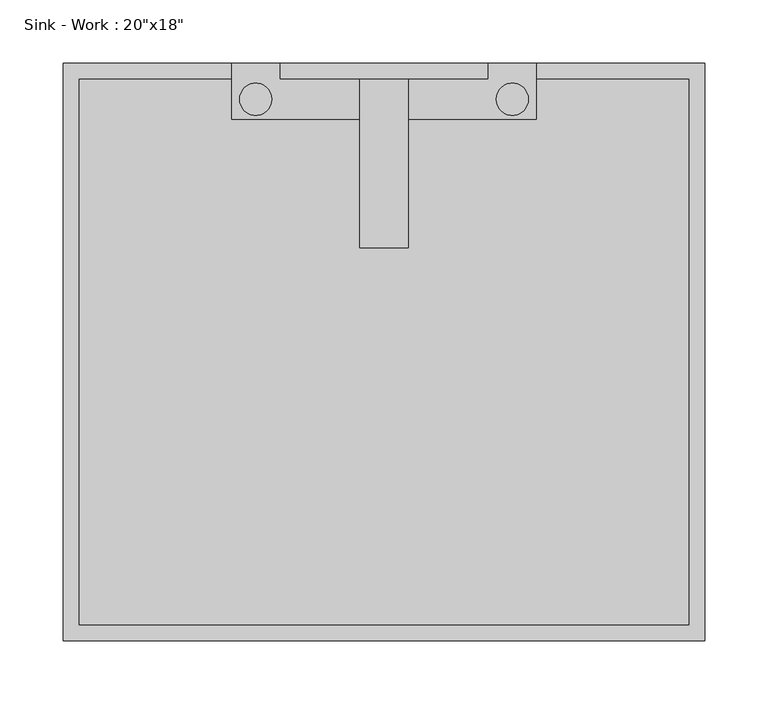
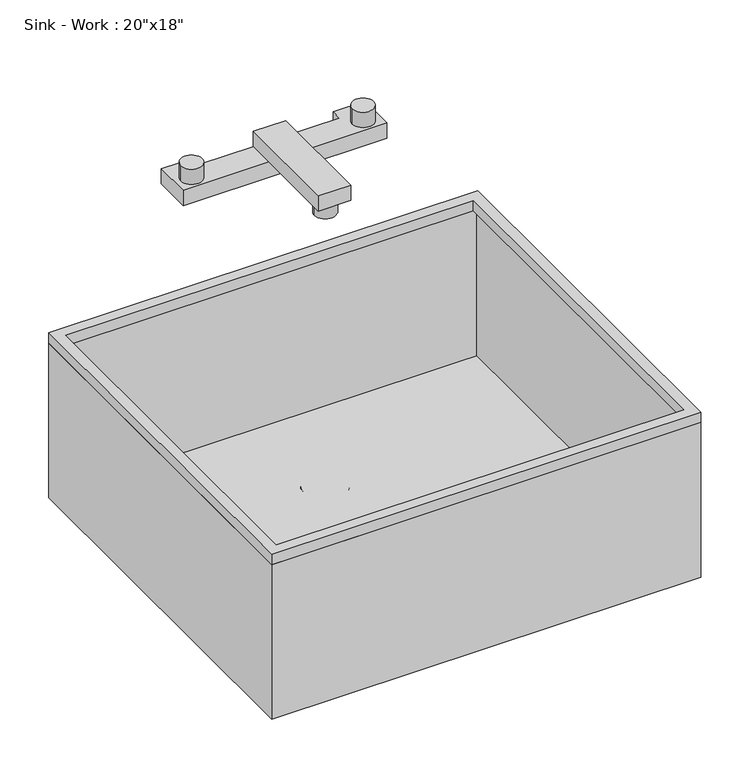
"""IFC4 building model written with IfcOpenShell, lengths in millimetres: flow terminal geometry."""

from ifc_helpers import new_model, si_unit, point, frame, frame_2d, origin, origin_with_axes, place, context, project, spatial, polyline, circle_curve, trimmed, segment, composite_curve, outline, extrude, faceted_brep, source, transform, mapped, element, save
from ifc_brep_helpers import plane_surface, cylinder_surface, advanced_brep


def flow_terminal_cce4e9d2(model_context):
    return source(origin(), model_context, "Body", "SolidModel", [
        extrude(outline(polyline([(254.0, 0.0), (254.0, -457.2), (-254.0, -457.2), (-254.0, 0.0), (254.0, 0.0)]), holes=[polyline([(241.3, -12.7), (-241.3, -12.7), (-241.3, -444.5), (241.3, -444.5), (241.3, -12.7)])]), frame((0.0, 0.0, 193.675), z_axis=(0.0, 0.0, 1.0), x_axis=(1.0, 0.0, 0.0)), (0.0, 0.0, 1.0), 12.7),
        faceted_brep([(254.0, 0.0, 193.675), (-254.0, 0.0, 193.675), (-254.0, -457.2, 193.675), (254.0, -457.2, 193.675), (250.825, -3.175, 193.675), (250.825, -454.025, 193.675), (-250.825, -454.025, 193.675), (-250.825, -3.175, 193.675), (254.0, 0.0, 0.0), (254.0, -457.2, 0.0), (-254.0, -457.2, 0.0), (-254.0, 0.0, 0.0), (250.825, -3.175, 3.175), (250.825, -454.025, 3.175), (-250.825, -454.025, 3.175), (-250.825, -3.175, 3.175)], [[[0, 1, 2, 3], [4, 5, 6, 7]], [[8, 9, 10, 11]], [[1, 0, 8, 11]], [[2, 1, 11, 10]], [[3, 2, 10, 9]], [[0, 3, 9, 8]], [[5, 4, 12, 13]], [[6, 5, 13, 14]], [[7, 6, 14, 15]], [[4, 7, 15, 12]], [[13, 12, 15, 14]]]),
        extrude(outline(composite_curve([segment(trimmed(circle_curve(frame_2d((0.0, -127.0)), 25.4), [point((-25.4, -127.0))], [point((25.4, -127.0))], False, "CARTESIAN"), True, "CONTINUOUS"), segment(trimmed(circle_curve(frame_2d((0.0, -127.0)), 25.4), [point((25.4, -127.0))], [point((-25.4, -127.0))], False, "CARTESIAN"), True, "CONTINUOUS")], self_intersect=False)), origin_with_axes(), (0.0, 0.0, 1.0), 3.175),
        advanced_brep(
        [(19.05, -12.7, 384.175), (-19.05, -12.7, 384.175), (-19.05, -146.05, 384.175), (19.05, -146.05, 384.175), (19.05, -146.05, 365.125), (-19.05, -146.05, 365.125), (-19.05, -44.45, 365.125), (19.05, -44.45, 365.125), (-12.7, -127.0, 365.125), (12.7, -127.0, 365.125), (19.05, -12.7, 365.125), (82.55, -12.7, 365.125), (82.55, -12.7, 346.075), (-82.55, -12.7, 346.075), (-82.55, -12.7, 365.125), (-19.05, -12.7, 365.125), (-12.7, -127.0, 346.075), (12.7, -127.0, 346.075), (-82.55, 0.0, 365.125), (-120.65, 0.0, 365.125), (-120.65, -44.45, 365.125), (-88.9, -28.575, 365.125), (-114.3, -28.575, 365.125), (120.65, -44.45, 365.125), (120.65, 0.0, 365.125), (82.55, 0.0, 365.125), (114.3, -28.575, 365.125), (88.9, -28.575, 365.125), (-82.55, 0.0, 346.075), (82.55, 0.0, 346.075), (120.65, 0.0, 346.075), (120.65, -44.45, 346.075), (-120.65, -44.45, 346.075), (-120.65, 0.0, 346.075), (-114.3, -28.575, 384.175), (-88.9, -28.575, 384.175), (88.9, -28.575, 384.175), (114.3, -28.575, 384.175)],
        [
            (0, 1),
            (1, 2),
            (2, 3),
            (3, 0),
            (4, 5),
            (5, 6),
            (6, 7),
            (7, 4),
            (8, 9, circle_curve(frame((0.0, -127.0, 365.125), z_axis=(0.0, 0.0, 1.0), x_axis=(1.0, 0.0, 0.0)), 12.7)),
            (9, 8, circle_curve(frame((0.0, -127.0, 365.125), z_axis=(0.0, 0.0, 1.0), x_axis=(1.0, 0.0, 0.0)), 12.7)),
            (0, 10),
            (10, 11),
            (11, 12),
            (12, 13),
            (13, 14),
            (14, 15),
            (15, 1),
            (15, 6),
            (5, 2),
            (4, 3),
            (7, 10),
            (16, 17, circle_curve(frame((0.0, -127.0, 346.075), z_axis=(0.0, 0.0, -1.0), x_axis=(1.0, 0.0, 0.0)), 12.7)),
            (17, 16, circle_curve(frame((0.0, -127.0, 346.075), z_axis=(0.0, 0.0, -1.0), x_axis=(1.0, 0.0, 0.0)), 12.7)),
            (17, 9),
            (8, 16),
            (18, 19),
            (19, 20),
            (20, 6),
            (14, 18),
            (21, 22, circle_curve(frame((-101.6, -28.575, 365.125), z_axis=(0.0, 0.0, -1.0), x_axis=(1.0, 0.0, 0.0)), 12.7)),
            (22, 21, circle_curve(frame((-101.6, -28.575, 365.125), z_axis=(0.0, 0.0, -1.0), x_axis=(1.0, 0.0, 0.0)), 12.7)),
            (23, 24),
            (24, 25),
            (25, 11),
            (7, 23),
            (26, 27, circle_curve(frame((101.6, -28.575, 365.125), z_axis=(0.0, 0.0, -1.0), x_axis=(1.0, 0.0, 0.0)), 12.7)),
            (27, 26, circle_curve(frame((101.6, -28.575, 365.125), z_axis=(0.0, 0.0, -1.0), x_axis=(1.0, 0.0, 0.0)), 12.7)),
            (28, 13),
            (12, 29),
            (29, 30),
            (30, 31),
            (31, 32),
            (32, 33),
            (33, 28),
            (18, 28),
            (33, 19),
            (32, 20),
            (31, 23),
            (30, 24),
            (29, 25),
            (34, 35, circle_curve(frame((-101.6, -28.575, 384.175), z_axis=(0.0, 0.0, 1.0), x_axis=(1.0, 0.0, 0.0)), 12.7)),
            (35, 34, circle_curve(frame((-101.6, -28.575, 384.175), z_axis=(0.0, 0.0, 1.0), x_axis=(1.0, 0.0, 0.0)), 12.7)),
            (36, 37, circle_curve(frame((101.6, -28.575, 384.175), z_axis=(0.0, 0.0, 1.0), x_axis=(1.0, 0.0, 0.0)), 12.7)),
            (37, 36, circle_curve(frame((101.6, -28.575, 384.175), z_axis=(0.0, 0.0, 1.0), x_axis=(1.0, 0.0, 0.0)), 12.7)),
            (34, 22),
            (21, 35),
            (36, 27),
            (26, 37),
        ],
        [
            plane_surface(frame((-19.05, -12.7, 384.175), z_axis=(0.0, 0.0, 1.0), x_axis=(-1.0, 0.0, 0.0))),
            plane_surface(frame((-19.05, -12.7, 365.125), z_axis=(0.0, 0.0, -1.0), x_axis=(1.0, 0.0, 0.0))),
            plane_surface(frame((19.05, -12.7, 384.175), z_axis=(0.0, 1.0, 0.0), x_axis=(0.0, 0.0, -1.0))),
            plane_surface(frame((-19.05, -12.7, 384.175), z_axis=(-1.0, 0.0, 0.0), x_axis=(0.0, 0.0, -1.0))),
            plane_surface(frame((-19.05, -146.05, 384.175), z_axis=(0.0, -1.0, 0.0), x_axis=(0.0, 0.0, -1.0))),
            plane_surface(frame((19.05, -146.05, 384.175), z_axis=(1.0, 0.0, 0.0), x_axis=(0.0, 0.0, -1.0))),
            plane_surface(frame((12.7, -127.0, 346.075), z_axis=(0.0, 0.0, -1.0), x_axis=(0.0, -1.0, 0.0))),
            cylinder_surface(frame((0.0, -127.0, 346.075), z_axis=(0.0, 0.0, 1.0), x_axis=(1.0, 0.0, 0.0)), 12.7),
            plane_surface(frame((-120.65, 0.0, 365.125), z_axis=(0.0, 0.0, 1.0), x_axis=(-1.0, 0.0, 0.0))),
            plane_surface(frame((-120.65, 0.0, 346.075), z_axis=(0.0, 0.0, -1.0), x_axis=(1.0, 0.0, 0.0))),
            plane_surface(frame((-82.55, 0.0, 365.125), z_axis=(0.0, 1.0, 0.0), x_axis=(0.0, 0.0, -1.0))),
            plane_surface(frame((-120.65, 0.0, 365.125), z_axis=(-1.0, 0.0, 0.0), x_axis=(0.0, 0.0, -1.0))),
            plane_surface(frame((-120.65, -44.45, 365.125), z_axis=(0.0, -1.0, 0.0), x_axis=(0.0, 0.0, -1.0))),
            plane_surface(frame((120.65, -44.45, 365.125), z_axis=(1.0, 0.0, 0.0), x_axis=(0.0, 0.0, -1.0))),
            plane_surface(frame((120.65, 0.0, 365.125), z_axis=(0.0, 1.0, 0.0), x_axis=(0.0, 0.0, -1.0))),
            plane_surface(frame((82.55, 0.0, 365.125), z_axis=(-1.0, 0.0, 0.0), x_axis=(0.0, 0.0, -1.0))),
            plane_surface(frame((-82.55, -12.7, 365.125), z_axis=(1.0, 0.0, 0.0), x_axis=(0.0, 0.0, -1.0))),
            plane_surface(frame((-88.9, -28.575, 384.175), z_axis=(0.0, 0.0, 1.0), x_axis=(0.0, 1.0, 0.0))),
            cylinder_surface(frame((-101.6, -28.575, 365.125), z_axis=(0.0, 0.0, 1.0), x_axis=(1.0, 0.0, 0.0)), 12.7),
            cylinder_surface(frame((101.6, -28.575, 0.0), z_axis=(0.0, 0.0, 1.0), x_axis=(1.0, 0.0, 0.0)), 12.7),
        ],
        [
            (0, [[1, 2, 3, 4]]),
            (1, [[5, 6, 7, 8], [9, 10]]),
            (2, [[-1, 11, 12, 13, 14, 15, 16, 17]]),
            (3, [[-2, -17, 18, -6, 19]]),
            (4, [[-3, -19, -5, 20]]),
            (5, [[-4, -20, -8, 21, -11]]),
            (6, [[22, 23]]),
            (7, [[-23, 24, -9, 25]]),
            (7, [[-22, -25, -10, -24]]),
            (8, [[26, 27, 28, -18, -16, 29], [30, 31]]),
            (8, [[32, 33, 34, -12, -21, 35], [36, 37]]),
            (9, [[38, -14, 39, 40, 41, 42, 43, 44]]),
            (10, [[-26, 45, -44, 46]]),
            (11, [[-27, -46, -43, 47]]),
            (12, [[-42, 48, -35, -7, -28, -47]]),
            (13, [[-32, -48, -41, 49]]),
            (14, [[-33, -49, -40, 50]]),
            (15, [[-34, -50, -39, -13]]),
            (16, [[-29, -15, -38, -45]]),
            (17, [[51, 52]]),
            (17, [[53, 54]]),
            (18, [[-51, 55, -30, 56]]),
            (18, [[-52, -56, -31, -55]]),
            (19, [[-53, 57, -36, 58]]),
            (19, [[-54, -58, -37, -57]]),
        ],
    ),
    ])


if __name__ == "__main__":
    model = new_model("IFC4")
    model_context = context("Model", 3, world=origin())
    ifc_project = project(units=[si_unit("LENGTHUNIT", "METRE", prefix="MILLI")], contexts=[model_context])
    site = spatial("IfcSite", under=ifc_project)
    building = spatial("IfcBuilding", under=site)
    placement = place(None, origin())
    flow_terminal_shape = flow_terminal_cce4e9d2(model_context)
    element("IfcFlowTerminal", 1, ObjectType="Sink - Work : 20\"x18\"", at=placement, inside=building, context=model_context, shape_type="MappedRepresentation", body=[
        mapped(flow_terminal_shape, transform((0.0, 0.0, 0.0), x_axis=(1.0, 0.0, 0.0), y_axis=(0.0, 1.0, 0.0), z_axis=(0.0, 0.0, 1.0))),
    ])
    save(model, "model.ifc")

# Revit data of these elements
# Type "Sink - Work : 20\"x18\""
#   WFU = 2
#   Sink Width = 1' - 6"
#   Sink Length = 1' - 8"
#   Sink Depth = 0' - 8"
#   Sanitary Radius = 3/4"
#   Sanitary Diameter = 1 1/2"
#   Hot Water Radius = 1/4"
#   Hot Water Diameter = 1/2"
#   HWFU = 2.25
#   Flow Pressure [instance default] = 8.00 psi
#   Faucet Height = 1' - 1 5/8"
#   Cold Water Radius = 1/4"
#   Cold Water Diameter = 1/2"
#   CWFU = 2.25
#   Sink Material = none
#   Faucet Material = none
#   Default Elevation = 0
